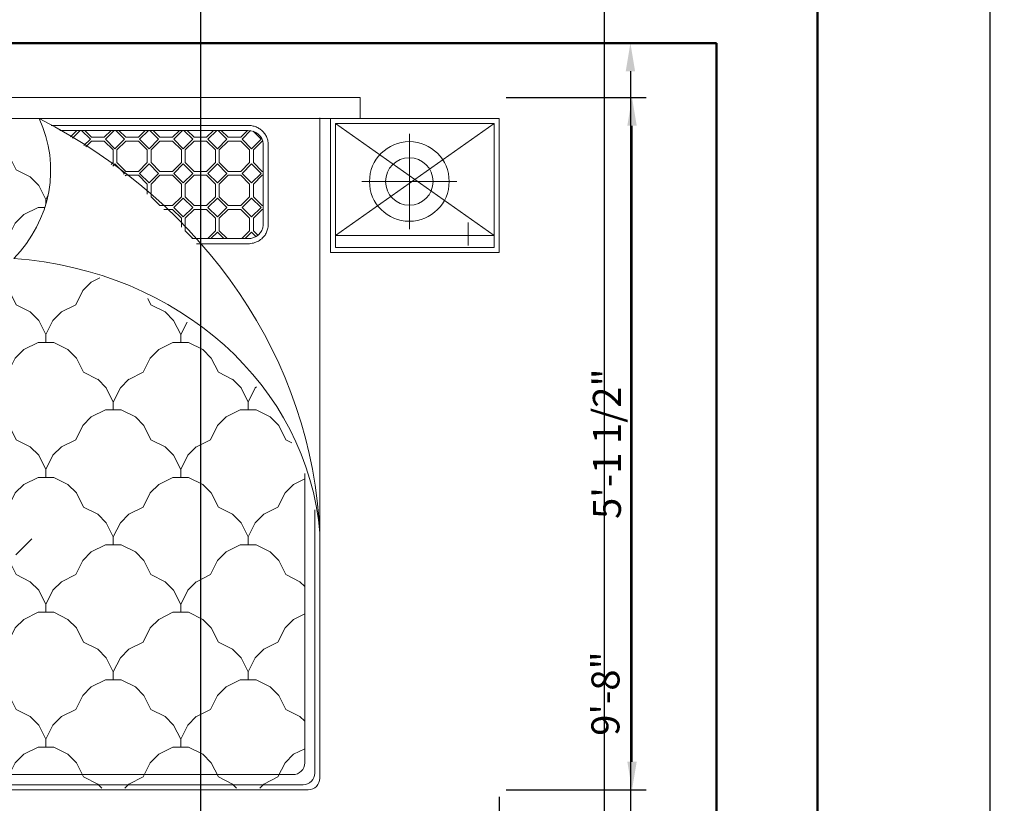
# Model space of a CAD drawing. Units: inches. Extents: x 2385 to 2740, y 1752 to 2305.
# Tile 6 of 15: x 2641 to 2729, y 1911 to 1981. Entities that reach past the tile are written whole.
import ezdxf

# ---------------------------------------------------------------- set-up
doc = ezdxf.new("R2010")
doc.units = ezdxf.units.IN
for name, color, linetype, lineweight in [('A-ANNO-DIMS', 2, 'Continuous', 18), ('A-FURN', 9, 'Continuous', 18), ('A-WALL', 7, 'Continuous', 50)]:
    doc.layers.add(name, color=color, linetype=linetype, lineweight=lineweight)
doc.styles.get("Standard").update_dxf_attribs({"font": 'arial.ttf'})
doc.dimstyles.new('Copy of ISO-25', dxfattribs={"dimtxt": 2.5, "dimasz": 2.5, "dimexe": 1.25, "dimexo": 0.625, "dimtad": 1, "dimdec": 1, "dimlunit": 4, "dimtxsty": 'Standard', "dimcen": 2.5, "dimadec": 0, "dimazin": 0, "dimtfac": 1, "dimtdec": 1, "dimtmove": 0, "dimatfit": 3, "dimfxl": 1, "dimarcsym": 0})

# ---------------------------------------------------------------- blocks, each defined once
blk = doc.blocks.new('A$C029D5C69')
for p, q in [((0.4164, 2.0693), (0.4164, 2.0066)), ((2.2315, 2.0693), (0.4164, 2.0693)), ((2.2315, 2.0066), (2.2315, 2.0693)), ((0, 1.606), (0, 2.0066)), ((0, 2.0066), (0.505, 2.0066)), ((0.4164, 2.0066), (2.2315, 2.0066)), ((0.505, 2.0066), (0.505, 1.606)), ((0.5252, 0.0351), (0.5252, 2.0066)), ((0.5403, 0.0502), (0.5403, 2.0066)), ((0.5706, 0.0805), (0.5706, 2.0066)), ((0.6869, 1.966), (0.6666, 2.0066)), ((0.7072, 2.0066), (0.6869, 1.966)), ((1.0902, 1.966), (1.0699, 2.0066)), ((1.1106, 2.0066), (1.0902, 1.966)), ((2.1114, 2.0087), (2.1114, 0.0351)), ((2.6479, 2.0066), (2.1429, 2.0066)), ((2.1429, 2.0066), (2.1429, 1.606)), ((2.6479, 1.606), (2.6479, 2.0066)), ((0.0151, 1.6211), (0.0151, 1.9915)), ((0.0151, 1.9915), (0.4899, 1.9915)), ((0.4899, 1.9915), (0.4899, 1.6211)), ((1.8954, 1.9865), (1.3081, 1.9865)), ((2.6328, 1.9915), (2.158, 1.9915)), ((2.158, 1.9915), (2.158, 1.6211)), ((2.6328, 1.6211), (2.6328, 1.9915)), ((0.2689, 1.9609), (0.2689, 1.6764)), ((0.6869, 1.9425), (0.6869, 1.966)), ((0.6869, 1.9425), (0.6869, 1.966)), ((1.0902, 1.9425), (1.0902, 1.966)), ((1.0902, 1.9425), (1.0902, 1.966)), ((1.8954, 1.9713), (1.3339, 1.9713)), ((1.3849, 1.9713), (1.3656, 1.952)), ((1.3945, 1.9713), (1.3714, 1.9483)), ((1.4249, 1.945), (1.3986, 1.9713)), ((1.4249, 1.945), (1.4059, 1.926)), ((1.4288, 1.9507), (1.4081, 1.9713)), ((1.4476, 1.9507), (1.4288, 1.9507)), ((1.4476, 1.9507), (1.4664, 1.9507)), ((1.487, 1.9713), (1.4664, 1.9507)), ((1.4966, 1.9713), (1.4703, 1.945)), ((1.4986, 1.9167), (1.4703, 1.945)), ((1.527, 1.945), (1.4986, 1.9167)), ((1.527, 1.945), (1.5007, 1.9713)), ((1.5309, 1.9507), (1.5102, 1.9713)), ((1.5497, 1.9507), (1.5309, 1.9507)), ((1.5497, 1.9507), (1.5685, 1.9507)), ((1.5891, 1.9713), (1.5685, 1.9507)), ((1.5987, 1.9713), (1.5724, 1.945)), ((1.6007, 1.9167), (1.5724, 1.945)), ((1.6291, 1.945), (1.6007, 1.9167)), ((1.6291, 1.945), (1.6028, 1.9713)), ((1.633, 1.9507), (1.6123, 1.9713)), ((1.6518, 1.9507), (1.633, 1.9507)), ((1.6518, 1.9507), (1.6706, 1.9507)), ((1.6912, 1.9713), (1.6706, 1.9507)), ((1.7008, 1.9713), (1.6745, 1.945)), ((1.7028, 1.9167), (1.6745, 1.945)), ((1.7312, 1.945), (1.7028, 1.9167)), ((1.7312, 1.945), (1.7049, 1.9713)), ((1.7351, 1.9507), (1.7144, 1.9713)), ((1.7539, 1.9507), (1.7351, 1.9507)), ((1.7539, 1.9507), (1.7727, 1.9507)), ((1.7933, 1.9713), (1.7727, 1.9507)), ((1.8029, 1.9713), (1.7766, 1.945)), ((1.8049, 1.9167), (1.7766, 1.945)), ((1.8333, 1.945), (1.8049, 1.9167)), ((1.8333, 1.945), (1.807, 1.9713)), ((1.8372, 1.9507), (1.8165, 1.9713)), ((1.856, 1.9507), (1.8372, 1.9507)), ((1.856, 1.9507), (1.8748, 1.9507)), ((1.8954, 1.9713), (1.8748, 1.9507)), ((1.9043, 1.9707), (1.8787, 1.945)), ((1.907, 1.9167), (1.8787, 1.945)), ((1.9354, 1.945), (1.907, 1.9167)), ((1.9354, 1.945), (1.9114, 1.969)), ((2.379, 1.9609), (2.379, 1.6764)), ((0.621, 1.9213), (0.5955, 1.8958)), ((0.6634, 1.9425), (0.621, 1.9213)), ((0.6634, 1.9425), (0.621, 1.9213)), ((0.6869, 1.9425), (0.6634, 1.9425)), ((0.6869, 1.9425), (0.7104, 1.9425)), ((0.7528, 1.9213), (0.7104, 1.9425)), ((0.7528, 1.9213), (0.7104, 1.9425)), ((0.7783, 1.8958), (0.7528, 1.9213)), ((1.0243, 1.9213), (0.9988, 1.8958)), ((1.0668, 1.9425), (1.0244, 1.9213)), ((1.0668, 1.9425), (1.0244, 1.9213)), ((1.0902, 1.9425), (1.0668, 1.9425)), ((1.0902, 1.9425), (1.1137, 1.9425)), ((1.1561, 1.9213), (1.1137, 1.9425)), ((1.1561, 1.9213), (1.1137, 1.9425)), ((1.1816, 1.8958), (1.1561, 1.9213)), ((1.4288, 1.9394), (1.4116, 1.9222)), ((1.4288, 1.9393), (1.4476, 1.9393)), ((1.4664, 1.9393), (1.4476, 1.9393)), ((1.493, 1.9128), (1.4664, 1.9394)), ((1.5309, 1.9394), (1.5043, 1.9128)), ((1.5309, 1.9393), (1.5497, 1.9393)), ((1.5685, 1.9393), (1.5497, 1.9393)), ((1.595, 1.9128), (1.5685, 1.9394)), ((1.633, 1.9394), (1.6064, 1.9128)), ((1.633, 1.9393), (1.6518, 1.9393)), ((1.6706, 1.9393), (1.6518, 1.9393)), ((1.6971, 1.9128), (1.6706, 1.9394)), ((1.7351, 1.9394), (1.7085, 1.9128)), ((1.7351, 1.9393), (1.7539, 1.9393)), ((1.7727, 1.9393), (1.7539, 1.9393)), ((1.7992, 1.9128), (1.7727, 1.9394)), ((1.8372, 1.9394), (1.8106, 1.9128)), ((1.8372, 1.9393), (1.856, 1.9393)), ((1.8748, 1.9393), (1.856, 1.9393)), ((1.9013, 1.9128), (1.8748, 1.9394)), ((1.9393, 1.9394), (1.9127, 1.9128)), ((1.9393, 1.9393), (1.9404, 1.9393)), ((1.9414, 1.688), (1.9414, 1.931)), ((1.9565, 1.688), (1.9565, 1.931)), ((0.5955, 1.8958), (0.5743, 1.8534)), ((0.7995, 1.8534), (0.7783, 1.8958)), ((0.9989, 1.8958), (0.9777, 1.8534)), ((1.2028, 1.8534), (1.1816, 1.8958)), ((1.493, 1.8752), (1.493, 1.9128)), ((1.5043, 1.8752), (1.5043, 1.9128)), ((1.595, 1.8752), (1.595, 1.9128)), ((1.6064, 1.8752), (1.6064, 1.9128)), ((1.6971, 1.8752), (1.6971, 1.9128)), ((1.7085, 1.8752), (1.7085, 1.9128)), ((1.7992, 1.8752), (1.7992, 1.9128)), ((1.8106, 1.8752), (1.8106, 1.9128)), ((1.9013, 1.8752), (1.9013, 1.9128)), ((1.9127, 1.8752), (1.9127, 1.9128)), ((1.493, 1.8752), (1.4867, 1.869)), ((1.4986, 1.8713), (1.4922, 1.8648)), ((1.527, 1.8429), (1.4986, 1.8713)), ((1.5309, 1.8486), (1.5043, 1.8752)), ((1.595, 1.8752), (1.5685, 1.8486)), ((1.6007, 1.8713), (1.5724, 1.8429)), ((1.6291, 1.8429), (1.6007, 1.8713)), ((1.633, 1.8486), (1.6064, 1.8752)), ((1.6971, 1.8752), (1.6706, 1.8486)), ((1.7028, 1.8713), (1.6745, 1.8429)), ((1.7312, 1.8429), (1.7028, 1.8713)), ((1.7351, 1.8486), (1.7085, 1.8752)), ((1.7992, 1.8752), (1.7727, 1.8486)), ((1.8049, 1.8713), (1.7766, 1.8429)), ((1.8333, 1.8429), (1.8049, 1.8713)), ((1.8372, 1.8486), (1.8106, 1.8752)), ((1.9013, 1.8752), (1.8748, 1.8486)), ((1.907, 1.8713), (1.8787, 1.8429)), ((1.9354, 1.8429), (1.907, 1.8713)), ((1.9393, 1.8486), (1.9127, 1.8752)), ((0.5743, 1.8534), (0.5706, 1.8515)), ((0.5743, 1.8534), (0.5706, 1.8515)), ((0.8419, 1.8322), (0.7995, 1.8534)), ((0.8419, 1.8322), (0.7995, 1.8534)), ((0.8674, 1.8067), (0.8419, 1.8322)), ((0.9352, 1.8322), (0.9097, 1.8067)), ((0.9777, 1.8534), (0.9353, 1.8322)), ((0.9777, 1.8534), (0.9353, 1.8322)), ((1.2452, 1.8322), (1.2028, 1.8534)), ((1.2452, 1.8322), (1.2028, 1.8534)), ((1.2707, 1.8067), (1.2452, 1.8322)), ((1.527, 1.8429), (1.5242, 1.8401)), ((1.5309, 1.8373), (1.5295, 1.8359)), ((1.5497, 1.8486), (1.5309, 1.8486)), ((1.5309, 1.8373), (1.5497, 1.8373)), ((1.5497, 1.8486), (1.5685, 1.8486)), ((1.5685, 1.8373), (1.5497, 1.8373)), ((1.595, 1.8107), (1.5685, 1.8373)), ((1.6007, 1.8146), (1.5724, 1.8429)), ((1.6291, 1.8429), (1.6007, 1.8146)), ((1.633, 1.8373), (1.6064, 1.8107)), ((1.6518, 1.8486), (1.633, 1.8486)), ((1.633, 1.8373), (1.6518, 1.8373)), ((1.6518, 1.8486), (1.6706, 1.8486)), ((1.6706, 1.8373), (1.6518, 1.8373)), ((1.6971, 1.8107), (1.6706, 1.8373)), ((1.7028, 1.8146), (1.6745, 1.8429)), ((1.7312, 1.8429), (1.7028, 1.8146)), ((1.7351, 1.8373), (1.7085, 1.8107)), ((1.7539, 1.8486), (1.7351, 1.8486)), ((1.7351, 1.8373), (1.7539, 1.8373)), ((1.7539, 1.8486), (1.7727, 1.8486)), ((1.7727, 1.8373), (1.7539, 1.8373)), ((1.7992, 1.8107), (1.7727, 1.8373)), ((1.8049, 1.8146), (1.7766, 1.8429)), ((1.8333, 1.8429), (1.8049, 1.8146)), ((1.8372, 1.8373), (1.8106, 1.8107)), ((1.856, 1.8486), (1.8372, 1.8486)), ((1.8372, 1.8373), (1.856, 1.8373)), ((1.856, 1.8486), (1.8748, 1.8486)), ((1.8748, 1.8373), (1.856, 1.8373)), ((1.9013, 1.8107), (1.8748, 1.8373)), ((1.907, 1.8146), (1.8787, 1.8429)), ((1.9354, 1.8429), (1.907, 1.8146)), ((1.9393, 1.8373), (1.9127, 1.8107)), ((1.9414, 1.8486), (1.9393, 1.8486)), ((1.9393, 1.8373), (1.9414, 1.8373)), ((0.1267, 1.8186), (0.4111, 1.8186)), ((0.8886, 1.7643), (0.8674, 1.8067)), ((0.9098, 1.8067), (0.8886, 1.7643)), ((1.2919, 1.7643), (1.2707, 1.8067)), ((1.595, 1.7806), (1.595, 1.8107)), ((1.6064, 1.7731), (1.6064, 1.8107)), ((1.6971, 1.7731), (1.6971, 1.8107)), ((1.7085, 1.7731), (1.7085, 1.8107)), ((1.7992, 1.7731), (1.7992, 1.8107)), ((1.8106, 1.7731), (1.8106, 1.8107)), ((1.9013, 1.7731), (1.9013, 1.8107)), ((1.9127, 1.7731), (1.9127, 1.8107)), ((2.2367, 1.8186), (2.5212, 1.8186)), ((1.2981, 1.7768), (1.2919, 1.7643)), ((1.633, 1.7465), (1.6064, 1.7731)), ((1.6971, 1.7731), (1.6706, 1.7465)), ((1.7028, 1.7692), (1.6745, 1.7408)), ((1.7312, 1.7408), (1.7028, 1.7692)), ((1.7351, 1.7465), (1.7085, 1.7731)), ((1.7992, 1.7731), (1.7727, 1.7465)), ((1.8049, 1.7692), (1.7766, 1.7408)), ((1.8333, 1.7408), (1.8049, 1.7692)), ((1.8372, 1.7465), (1.8106, 1.7731)), ((1.9013, 1.7731), (1.8748, 1.7465)), ((1.907, 1.7692), (1.8787, 1.7408)), ((1.9354, 1.7408), (1.907, 1.7692)), ((1.9393, 1.7465), (1.9127, 1.7731)), ((0.8651, 1.7408), (0.8227, 1.7196)), ((0.8651, 1.7408), (0.8227, 1.7196)), ((0.912, 1.7408), (0.8651, 1.7408)), ((0.8886, 1.7408), (0.8886, 1.7643)), ((0.9544, 1.7196), (0.912, 1.7408)), ((0.9544, 1.7196), (0.912, 1.7408)), ((1.2684, 1.7408), (1.226, 1.7196)), ((1.2684, 1.7408), (1.226, 1.7196)), ((1.2885, 1.7408), (1.2684, 1.7408)), ((1.2919, 1.7519), (1.2919, 1.7643)), ((1.6518, 1.7465), (1.633, 1.7465)), ((1.6518, 1.7465), (1.6706, 1.7465)), ((1.7028, 1.7125), (1.6745, 1.7408)), ((1.7312, 1.7408), (1.7028, 1.7125)), ((1.7539, 1.7465), (1.7351, 1.7465)), ((1.7539, 1.7465), (1.7727, 1.7465)), ((1.8049, 1.7125), (1.7766, 1.7408)), ((1.8333, 1.7408), (1.8049, 1.7125)), ((1.856, 1.7465), (1.8372, 1.7465)), ((1.856, 1.7465), (1.8748, 1.7465)), ((1.907, 1.7125), (1.8787, 1.7408)), ((1.9354, 1.7408), (1.907, 1.7125)), ((1.9414, 1.7465), (1.9393, 1.7465)), ((0.8227, 1.7196), (0.7972, 1.6941)), ((0.98, 1.6941), (0.9545, 1.7196)), ((1.226, 1.7196), (1.2005, 1.6941)), ((1.6443, 1.7352), (1.6518, 1.7352)), ((1.6706, 1.7352), (1.6518, 1.7352)), ((1.6971, 1.7086), (1.6706, 1.7352)), ((1.6971, 1.682), (1.6971, 1.7086)), ((1.7351, 1.7352), (1.7085, 1.7086)), ((1.7085, 1.671), (1.7085, 1.7086)), ((1.7351, 1.7352), (1.7539, 1.7352)), ((1.7727, 1.7352), (1.7539, 1.7352)), ((1.7992, 1.7086), (1.7727, 1.7352)), ((1.7992, 1.671), (1.7992, 1.7086)), ((1.8372, 1.7352), (1.8106, 1.7086)), ((1.8106, 1.671), (1.8106, 1.7086)), ((1.8372, 1.7352), (1.856, 1.7352)), ((1.8748, 1.7352), (1.856, 1.7352)), ((1.9013, 1.7086), (1.8748, 1.7352)), ((1.9013, 1.671), (1.9013, 1.7086)), ((1.9393, 1.7352), (1.9127, 1.7086)), ((1.9127, 1.671), (1.9127, 1.7086)), ((1.9393, 1.7352), (1.9414, 1.7352)), ((0.5766, 1.6941), (0.5706, 1.7002)), ((0.5978, 1.6517), (0.5766, 1.6941)), ((0.7972, 1.6941), (0.776, 1.6517)), ((1.0011, 1.6517), (0.9799, 1.6941)), ((1.2005, 1.6941), (1.1793, 1.6517)), ((2.5551, 1.6275), (2.5551, 1.696)), ((0.6402, 1.6305), (0.5978, 1.6517)), ((0.6402, 1.6305), (0.5978, 1.6517)), ((0.776, 1.6517), (0.7336, 1.6305)), ((0.776, 1.6517), (0.7336, 1.6305)), ((1.0435, 1.6305), (1.0011, 1.6517)), ((1.0435, 1.6305), (1.0011, 1.6517)), ((1.1793, 1.6517), (1.1369, 1.6305)), ((1.1793, 1.6517), (1.1369, 1.6305)), ((1.7318, 1.6477), (1.7085, 1.671)), ((1.7992, 1.671), (1.7759, 1.6477)), ((1.8049, 1.6671), (1.7855, 1.6477)), ((1.8244, 1.6477), (1.8049, 1.6671)), ((1.8339, 1.6477), (1.8106, 1.671)), ((1.9013, 1.671), (1.878, 1.6477)), ((1.907, 1.6671), (1.8876, 1.6477)), ((1.9202, 1.6539), (1.907, 1.6671)), ((1.926, 1.6577), (1.9127, 1.671)), ((0.4899, 1.6211), (0.0151, 1.6211)), ((0.6657, 1.605), (0.6402, 1.6305)), ((0.7336, 1.6305), (0.7081, 1.605)), ((1.0691, 1.605), (1.0436, 1.6305)), ((1.1369, 1.6305), (1.1114, 1.605)), ((1.8961, 1.6477), (1.7289, 1.6477)), ((1.8961, 1.6325), (1.7422, 1.6325)), ((2.158, 1.6211), (2.6328, 1.6211)), ((0.505, 1.606), (0, 1.606)), ((0.6869, 1.5626), (0.6657, 1.605)), ((0.7081, 1.605), (0.6869, 1.5626)), ((1.0902, 1.5626), (1.069, 1.605)), ((1.1114, 1.605), (1.0902, 1.5626)), ((2.1429, 1.606), (2.6479, 1.606)), ((0.6869, 1.5392), (0.6869, 1.5626)), ((0.6869, 1.5392), (0.6869, 1.5626)), ((1.0902, 1.5392), (1.0902, 1.5626)), ((1.0902, 1.5392), (1.0902, 1.5626)), ((0.6634, 1.5391), (0.621, 1.5179)), ((0.6634, 1.5391), (0.621, 1.5179)), ((0.6869, 1.5392), (0.6634, 1.5392)), ((0.6869, 1.5392), (0.7104, 1.5392)), ((0.7528, 1.5179), (0.7104, 1.5391)), ((0.7528, 1.5179), (0.7104, 1.5391)), ((1.0668, 1.5391), (1.0244, 1.5179)), ((1.0668, 1.5391), (1.0244, 1.5179)), ((1.0902, 1.5392), (1.0668, 1.5392)), ((1.0902, 1.5392), (1.1137, 1.5392)), ((1.1561, 1.5179), (1.1137, 1.5391)), ((1.1561, 1.5179), (1.1137, 1.5391)), ((0.621, 1.5179), (0.5955, 1.4924)), ((0.7783, 1.4924), (0.7528, 1.5179)), ((1.0243, 1.5179), (0.9988, 1.4924)), ((1.1816, 1.4924), (1.1561, 1.5179)), ((1.4277, 1.5179), (1.4022, 1.4924)), ((1.4534, 1.5308), (1.4277, 1.5179)), ((1.4534, 1.5308), (1.4277, 1.5179)), ((0.5955, 1.4925), (0.5743, 1.4501)), ((0.7995, 1.4501), (0.7783, 1.4925)), ((0.9989, 1.4925), (0.9777, 1.4501)), ((1.2028, 1.4501), (1.1816, 1.4925)), ((1.4022, 1.4925), (1.381, 1.4501)), ((0.5743, 1.45), (0.5706, 1.4481)), ((0.5743, 1.45), (0.5706, 1.4481)), ((0.8419, 1.4288), (0.7995, 1.45)), ((0.8419, 1.4288), (0.7995, 1.45)), ((0.9777, 1.45), (0.9353, 1.4288)), ((0.9777, 1.45), (0.9353, 1.4288)), ((1.2452, 1.4288), (1.2028, 1.45)), ((1.2452, 1.4288), (1.2028, 1.45)), ((1.381, 1.45), (1.3386, 1.4288)), ((1.381, 1.45), (1.3386, 1.4288)), ((1.6062, 1.4501), (1.5966, 1.4692)), ((1.6486, 1.4288), (1.6062, 1.45)), ((1.6486, 1.4288), (1.6062, 1.45)), ((0.8674, 1.4033), (0.8419, 1.4288)), ((0.9352, 1.4288), (0.9097, 1.4033)), ((1.2707, 1.4033), (1.2452, 1.4288)), ((1.3386, 1.4288), (1.3131, 1.4033)), ((1.6741, 1.4033), (1.6486, 1.4288)), ((0.5403, 1.4117), (0.5706, 1.4117)), ((0.8886, 1.361), (0.8674, 1.4034)), ((0.9098, 1.4034), (0.8886, 1.361)), ((1.2919, 1.361), (1.2707, 1.4034)), ((1.3131, 1.4034), (1.2919, 1.361)), ((1.6953, 1.361), (1.6741, 1.4034)), ((1.714, 1.3984), (1.6953, 1.361)), ((0.8886, 1.3375), (0.8886, 1.3609)), ((1.2919, 1.3375), (1.2919, 1.3609)), ((1.6953, 1.3375), (1.6953, 1.3609)), ((0.8651, 1.3374), (0.8227, 1.3162)), ((0.8651, 1.3374), (0.8227, 1.3162)), ((0.912, 1.3375), (0.8651, 1.3375)), ((0.9544, 1.3162), (0.912, 1.3374)), ((0.9544, 1.3162), (0.912, 1.3374)), ((1.2684, 1.3374), (1.226, 1.3162)), ((1.2684, 1.3374), (1.226, 1.3162)), ((1.3154, 1.3375), (1.2684, 1.3375)), ((1.3578, 1.3162), (1.3154, 1.3374)), ((1.3578, 1.3162), (1.3154, 1.3374)), ((1.6718, 1.3374), (1.6294, 1.3162)), ((1.6718, 1.3374), (1.6294, 1.3162)), ((1.7187, 1.3375), (1.6718, 1.3375)), ((1.7611, 1.3162), (1.7187, 1.3374)), ((1.7611, 1.3162), (1.7187, 1.3374)), ((0.5766, 1.2908), (0.5706, 1.2968)), ((0.8227, 1.3163), (0.7972, 1.2908)), ((0.98, 1.2908), (0.9545, 1.3163)), ((1.226, 1.3163), (1.2005, 1.2908)), ((1.3833, 1.2908), (1.3578, 1.3163)), ((1.6294, 1.3163), (1.6039, 1.2908)), ((1.7867, 1.2908), (1.7611, 1.3163)), ((0.5978, 1.2484), (0.5766, 1.2908)), ((0.7972, 1.2908), (0.776, 1.2484)), ((1.0011, 1.2484), (0.9799, 1.2908)), ((1.2005, 1.2908), (1.1793, 1.2484)), ((1.4045, 1.2484), (1.3833, 1.2908)), ((1.6039, 1.2908), (1.5827, 1.2484)), ((1.8078, 1.2484), (1.7866, 1.2908)), ((0.6402, 1.2271), (0.5978, 1.2483)), ((0.6402, 1.2271), (0.5978, 1.2483)), ((0.776, 1.2483), (0.7336, 1.2271)), ((0.776, 1.2483), (0.7336, 1.2271)), ((1.0435, 1.2271), (1.0011, 1.2483)), ((1.0435, 1.2271), (1.0011, 1.2483)), ((1.1793, 1.2483), (1.1369, 1.2271)), ((1.1793, 1.2483), (1.1369, 1.2271)), ((1.4469, 1.2271), (1.4045, 1.2483)), ((1.4469, 1.2271), (1.4045, 1.2483)), ((1.5827, 1.2483), (1.5403, 1.2271)), ((1.5827, 1.2483), (1.5403, 1.2271)), ((1.8502, 1.2271), (1.8078, 1.2483)), ((1.8502, 1.2271), (1.8078, 1.2483)), ((0.5403, 1.21), (0.5706, 1.21)), ((0.6657, 1.2017), (0.6402, 1.2272)), ((0.7336, 1.2272), (0.7081, 1.2017)), ((1.0691, 1.2017), (1.0436, 1.2272)), ((1.1369, 1.2272), (1.1114, 1.2017)), ((1.4724, 1.2017), (1.4469, 1.2272)), ((1.5403, 1.2272), (1.5148, 1.2017)), ((1.8758, 1.2017), (1.8503, 1.2272)), ((0.6869, 1.1593), (0.6657, 1.2017)), ((0.7081, 1.2017), (0.6869, 1.1593)), ((1.0902, 1.1593), (1.069, 1.2017)), ((1.1114, 1.2017), (1.0902, 1.1593)), ((1.4936, 1.1593), (1.4724, 1.2017)), ((1.5148, 1.2017), (1.4936, 1.1593)), ((1.8969, 1.1593), (1.8757, 1.2017)), ((1.9181, 1.2017), (1.8969, 1.1593)), ((1.9215, 1.2051), (1.9181, 1.2017)), ((0.6869, 1.1358), (0.6869, 1.1593)), ((0.6869, 1.1358), (0.6869, 1.1593)), ((1.0902, 1.1358), (1.0902, 1.1593)), ((1.0902, 1.1358), (1.0902, 1.1593)), ((1.4936, 1.1358), (1.4936, 1.1593)), ((1.4936, 1.1358), (1.4936, 1.1593)), ((1.8969, 1.1358), (1.8969, 1.1593)), ((1.8969, 1.1358), (1.8969, 1.1593)), ((0.6634, 1.1358), (0.621, 1.1146)), ((0.6634, 1.1358), (0.621, 1.1146)), ((0.6869, 1.1358), (0.6634, 1.1358)), ((0.6869, 1.1358), (0.7104, 1.1358)), ((0.7528, 1.1146), (0.7104, 1.1358)), ((0.7528, 1.1146), (0.7104, 1.1358)), ((1.0668, 1.1358), (1.0244, 1.1146)), ((1.0668, 1.1358), (1.0244, 1.1146)), ((1.0902, 1.1358), (1.0668, 1.1358)), ((1.0902, 1.1358), (1.1137, 1.1358)), ((1.1561, 1.1146), (1.1137, 1.1358)), ((1.1561, 1.1146), (1.1137, 1.1358)), ((1.4701, 1.1358), (1.4277, 1.1146)), ((1.4701, 1.1358), (1.4277, 1.1146)), ((1.4936, 1.1358), (1.4701, 1.1358)), ((1.4936, 1.1358), (1.5171, 1.1358)), ((1.5595, 1.1146), (1.5171, 1.1358)), ((1.5595, 1.1146), (1.5171, 1.1358)), ((1.8735, 1.1358), (1.8311, 1.1146)), ((1.8735, 1.1358), (1.8311, 1.1146)), ((1.8969, 1.1358), (1.8735, 1.1358)), ((1.8969, 1.1358), (1.9204, 1.1358)), ((1.9628, 1.1146), (1.9204, 1.1358)), ((1.9628, 1.1146), (1.9204, 1.1358)), ((0.621, 1.1146), (0.5955, 1.0891)), ((0.7783, 1.0891), (0.7528, 1.1146)), ((1.0243, 1.1146), (0.9988, 1.0891)), ((1.1816, 1.0891), (1.1561, 1.1146)), ((1.4277, 1.1146), (1.4022, 1.0891)), ((1.585, 1.0891), (1.5595, 1.1146)), ((1.831, 1.1146), (1.8055, 1.0891)), ((1.9883, 1.0891), (1.9628, 1.1146)), ((0.5955, 1.0891), (0.5743, 1.0467)), ((0.7995, 1.0467), (0.7783, 1.0891)), ((0.9989, 1.0891), (0.9777, 1.0467)), ((1.2028, 1.0467), (1.1816, 1.0891)), ((1.4022, 1.0891), (1.381, 1.0467)), ((1.6062, 1.0467), (1.585, 1.0891)), ((1.8056, 1.0891), (1.7844, 1.0467)), ((2.0095, 1.0467), (1.9883, 1.0891)), ((0.5743, 1.0467), (0.5706, 1.0448)), ((0.5743, 1.0467), (0.5706, 1.0448)), ((0.8419, 1.0255), (0.7995, 1.0467)), ((0.8419, 1.0255), (0.7995, 1.0467)), ((0.9777, 1.0467), (0.9353, 1.0255)), ((0.9777, 1.0467), (0.9353, 1.0255)), ((1.2452, 1.0255), (1.2028, 1.0467)), ((1.2452, 1.0255), (1.2028, 1.0467)), ((1.381, 1.0467), (1.3386, 1.0255)), ((1.381, 1.0467), (1.3386, 1.0255)), ((1.6486, 1.0255), (1.6062, 1.0467)), ((1.6486, 1.0255), (1.6062, 1.0467)), ((1.7844, 1.0467), (1.742, 1.0255)), ((1.7844, 1.0467), (1.742, 1.0255)), ((2.0276, 1.0376), (2.0095, 1.0467)), ((2.0276, 1.0376), (2.0095, 1.0467)), ((0.8674, 1), (0.8419, 1.0255)), ((0.9352, 1.0255), (0.9097, 1)), ((1.2707, 1), (1.2452, 1.0255)), ((1.3386, 1.0255), (1.3131, 1)), ((1.6741, 1), (1.6486, 1.0255)), ((1.7419, 1.0255), (1.7164, 1)), ((0.8886, 0.9576), (0.8674, 1)), ((0.9098, 1), (0.8886, 0.9576)), ((1.2919, 0.9576), (1.2707, 1)), ((1.3131, 1), (1.2919, 0.9576)), ((1.6953, 0.9576), (1.6741, 1)), ((1.7165, 1), (1.6953, 0.9576)), ((0.8886, 0.9341), (0.8886, 0.9576)), ((1.2919, 0.9341), (1.2919, 0.9576)), ((1.6953, 0.9341), (1.6953, 0.9576)), ((2.066, 0.9457), (2.066, 0.0805)), ((0.8651, 0.9341), (0.8227, 0.9129)), ((0.8651, 0.9341), (0.8227, 0.9129)), ((0.912, 0.9341), (0.8651, 0.9341)), ((0.9544, 0.9129), (0.912, 0.9341)), ((0.9544, 0.9129), (0.912, 0.9341)), ((1.2684, 0.9341), (1.226, 0.9129)), ((1.2684, 0.9341), (1.226, 0.9129)), ((1.3154, 0.9341), (1.2684, 0.9341)), ((1.3578, 0.9129), (1.3154, 0.9341)), ((1.3578, 0.9129), (1.3154, 0.9341)), ((1.6718, 0.9341), (1.6294, 0.9129)), ((1.6718, 0.9341), (1.6294, 0.9129)), ((1.7187, 0.9341), (1.6718, 0.9341)), ((1.7611, 0.9129), (1.7187, 0.9341)), ((1.7611, 0.9129), (1.7187, 0.9341)), ((2.066, 0.9295), (2.0327, 0.9129)), ((2.066, 0.9295), (2.0327, 0.9129)), ((0.5766, 0.8874), (0.5706, 0.8935)), ((0.5978, 0.845), (0.5766, 0.8874)), ((0.7972, 0.8874), (0.776, 0.845)), ((0.8227, 0.9129), (0.7972, 0.8874)), ((0.98, 0.8874), (0.9545, 0.9129)), ((1.0011, 0.845), (0.9799, 0.8874)), ((1.2005, 0.8874), (1.1793, 0.845)), ((1.226, 0.9129), (1.2005, 0.8874)), ((1.3833, 0.8874), (1.3578, 0.9129)), ((1.4045, 0.845), (1.3833, 0.8874)), ((1.6039, 0.8874), (1.5827, 0.845)), ((1.6294, 0.9129), (1.6039, 0.8874)), ((1.7867, 0.8874), (1.7611, 0.9129)), ((1.8078, 0.845), (1.7866, 0.8874)), ((2.0072, 0.8874), (1.986, 0.845)), ((2.0327, 0.9129), (2.0072, 0.8874)), ((0.6402, 0.8238), (0.5978, 0.845)), ((0.6402, 0.8238), (0.5978, 0.845)), ((0.776, 0.845), (0.7336, 0.8238)), ((0.776, 0.845), (0.7336, 0.8238)), ((1.0435, 0.8238), (1.0011, 0.845)), ((1.0435, 0.8238), (1.0011, 0.845)), ((1.1793, 0.845), (1.1369, 0.8238)), ((1.1793, 0.845), (1.1369, 0.8238)), ((1.4469, 0.8238), (1.4045, 0.845)), ((1.4469, 0.8238), (1.4045, 0.845)), ((1.5827, 0.845), (1.5403, 0.8238)), ((1.5827, 0.845), (1.5403, 0.8238)), ((1.8502, 0.8238), (1.8078, 0.845)), ((1.8502, 0.8238), (1.8078, 0.845)), ((1.986, 0.845), (1.9436, 0.8238)), ((1.986, 0.845), (1.9436, 0.8238)), ((2.0962, 0.8369), (2.0962, 0.0502)), ((0.6657, 0.7983), (0.6402, 0.8238)), ((0.6869, 0.7559), (0.6657, 0.7983)), ((0.7081, 0.7983), (0.6869, 0.7559)), ((0.7336, 0.8238), (0.7081, 0.7983)), ((1.0691, 0.7983), (1.0436, 0.8238)), ((1.0902, 0.7559), (1.069, 0.7983)), ((1.1114, 0.7983), (1.0902, 0.7559)), ((1.1369, 0.8238), (1.1114, 0.7983)), ((1.4724, 0.7983), (1.4469, 0.8238)), ((1.4936, 0.7559), (1.4724, 0.7983)), ((1.5148, 0.7983), (1.4936, 0.7559)), ((1.5403, 0.8238), (1.5148, 0.7983)), ((1.8758, 0.7983), (1.8503, 0.8238)), ((1.8969, 0.7559), (1.8757, 0.7983)), ((1.9181, 0.7983), (1.8969, 0.7559)), ((1.9436, 0.8238), (1.9181, 0.7983)), ((0.6869, 0.7325), (0.6869, 0.7559)), ((0.6869, 0.7325), (0.6869, 0.7559)), ((1.0902, 0.7325), (1.0902, 0.7559)), ((1.0902, 0.7325), (1.0902, 0.7559)), ((1.2024, 0.7028), (1.2503, 0.7507)), ((1.4936, 0.7325), (1.4936, 0.7559)), ((1.4936, 0.7325), (1.4936, 0.7559)), ((1.8969, 0.7325), (1.8969, 0.7559)), ((1.8969, 0.7325), (1.8969, 0.7559)), ((0.621, 0.7113), (0.5955, 0.6858)), ((0.6634, 0.7324), (0.621, 0.7112)), ((0.6634, 0.7324), (0.621, 0.7112)), ((0.6869, 0.7325), (0.6634, 0.7325)), ((0.6869, 0.7325), (0.7104, 0.7325)), ((0.7528, 0.7112), (0.7104, 0.7324)), ((0.7528, 0.7112), (0.7104, 0.7324)), ((0.7783, 0.6858), (0.7528, 0.7113)), ((1.0243, 0.7113), (0.9988, 0.6858)), ((1.0668, 0.7324), (1.0244, 0.7112)), ((1.0668, 0.7324), (1.0244, 0.7112)), ((1.0902, 0.7325), (1.0668, 0.7325)), ((1.0902, 0.7325), (1.1137, 0.7325)), ((1.1561, 0.7112), (1.1137, 0.7324)), ((1.1561, 0.7112), (1.1137, 0.7324)), ((1.1816, 0.6858), (1.1561, 0.7113)), ((1.4277, 0.7113), (1.4022, 0.6858)), ((1.4701, 0.7324), (1.4277, 0.7112)), ((1.4701, 0.7324), (1.4277, 0.7112)), ((1.4936, 0.7325), (1.4701, 0.7325)), ((1.4936, 0.7325), (1.5171, 0.7325)), ((1.5595, 0.7112), (1.5171, 0.7324)), ((1.5595, 0.7112), (1.5171, 0.7324)), ((1.585, 0.6858), (1.5595, 0.7113)), ((1.831, 0.7113), (1.8055, 0.6858)), ((1.8735, 0.7324), (1.8311, 0.7112)), ((1.8735, 0.7324), (1.8311, 0.7112)), ((1.8969, 0.7325), (1.8735, 0.7325)), ((1.8969, 0.7325), (1.9204, 0.7325)), ((1.9628, 0.7112), (1.9204, 0.7324)), ((1.9628, 0.7112), (1.9204, 0.7324)), ((1.9883, 0.6858), (1.9628, 0.7113)), ((0.5955, 0.6858), (0.5743, 0.6434)), ((0.7995, 0.6434), (0.7783, 0.6858)), ((0.9989, 0.6858), (0.9777, 0.6434)), ((1.2028, 0.6434), (1.1816, 0.6858)), ((1.4022, 0.6858), (1.381, 0.6434)), ((1.6062, 0.6434), (1.585, 0.6858)), ((1.8056, 0.6858), (1.7844, 0.6434)), ((2.0095, 0.6434), (1.9883, 0.6858)), ((0.5743, 0.6433), (0.5706, 0.6414)), ((0.5743, 0.6433), (0.5706, 0.6414)), ((0.8419, 0.6221), (0.7995, 0.6433)), ((0.8419, 0.6221), (0.7995, 0.6433)), ((0.8674, 0.5967), (0.8419, 0.6222)), ((0.9352, 0.6222), (0.9097, 0.5967)), ((0.9777, 0.6433), (0.9353, 0.6221)), ((0.9777, 0.6433), (0.9353, 0.6221)), ((1.2452, 0.6221), (1.2028, 0.6433)), ((1.2452, 0.6221), (1.2028, 0.6433)), ((1.2707, 0.5967), (1.2452, 0.6222)), ((1.3386, 0.6222), (1.3131, 0.5967)), ((1.381, 0.6433), (1.3386, 0.6221)), ((1.381, 0.6433), (1.3386, 0.6221)), ((1.6486, 0.6221), (1.6062, 0.6433)), ((1.6486, 0.6221), (1.6062, 0.6433)), ((1.6741, 0.5967), (1.6486, 0.6222)), ((1.7419, 0.6222), (1.7164, 0.5967)), ((1.7844, 0.6433), (1.742, 0.6221)), ((1.7844, 0.6433), (1.742, 0.6221)), ((2.0519, 0.6221), (2.0095, 0.6433)), ((2.0519, 0.6221), (2.0095, 0.6433)), ((2.066, 0.6081), (2.0519, 0.6222)), ((0.8886, 0.5543), (0.8674, 0.5967)), ((0.9098, 0.5967), (0.8886, 0.5543)), ((1.2919, 0.5543), (1.2707, 0.5967)), ((1.3131, 0.5967), (1.2919, 0.5543)), ((1.6953, 0.5543), (1.6741, 0.5967)), ((1.7165, 0.5967), (1.6953, 0.5543)), ((0.8651, 0.5308), (0.8227, 0.5096)), ((0.8651, 0.5308), (0.8227, 0.5096)), ((0.912, 0.5308), (0.8651, 0.5308)), ((0.8886, 0.5308), (0.8886, 0.5543)), ((0.9544, 0.5096), (0.912, 0.5308)), ((0.9544, 0.5096), (0.912, 0.5308)), ((1.2684, 0.5308), (1.226, 0.5096)), ((1.2684, 0.5308), (1.226, 0.5096)), ((1.3154, 0.5308), (1.2684, 0.5308)), ((1.2919, 0.5308), (1.2919, 0.5543)), ((1.3578, 0.5096), (1.3154, 0.5308)), ((1.3578, 0.5096), (1.3154, 0.5308)), ((1.6718, 0.5308), (1.6294, 0.5096)), ((1.6718, 0.5308), (1.6294, 0.5096)), ((1.7187, 0.5308), (1.6718, 0.5308)), ((1.6953, 0.5308), (1.6953, 0.5543)), ((1.7611, 0.5096), (1.7187, 0.5308)), ((1.7611, 0.5096), (1.7187, 0.5308)), ((0.8227, 0.5096), (0.7972, 0.4841)), ((0.98, 0.4841), (0.9545, 0.5096)), ((1.226, 0.5096), (1.2005, 0.4841)), ((1.3833, 0.4841), (1.3578, 0.5096)), ((1.6294, 0.5096), (1.6039, 0.4841)), ((1.7867, 0.4841), (1.7611, 0.5096)), ((2.0327, 0.5096), (2.0072, 0.4841)), ((2.066, 0.5262), (2.0327, 0.5096)), ((2.066, 0.5262), (2.0327, 0.5096)), ((0.5766, 0.4841), (0.5706, 0.4901)), ((0.5978, 0.4417), (0.5766, 0.4841)), ((0.7972, 0.4841), (0.776, 0.4417)), ((1.0011, 0.4417), (0.9799, 0.4841)), ((1.2005, 0.4841), (1.1793, 0.4417)), ((1.4045, 0.4417), (1.3833, 0.4841)), ((1.6039, 0.4841), (1.5827, 0.4417)), ((1.8078, 0.4417), (1.7866, 0.4841)), ((2.0072, 0.4841), (1.986, 0.4417)), ((0.6402, 0.4205), (0.5978, 0.4417)), ((0.6402, 0.4205), (0.5978, 0.4417)), ((0.6657, 0.395), (0.6402, 0.4205)), ((0.7336, 0.4205), (0.7081, 0.395)), ((0.776, 0.4417), (0.7336, 0.4205)), ((0.776, 0.4417), (0.7336, 0.4205)), ((1.0435, 0.4205), (1.0011, 0.4417)), ((1.0435, 0.4205), (1.0011, 0.4417)), ((1.0691, 0.395), (1.0436, 0.4205)), ((1.1369, 0.4205), (1.1114, 0.395)), ((1.1793, 0.4417), (1.1369, 0.4205)), ((1.1793, 0.4417), (1.1369, 0.4205)), ((1.4469, 0.4205), (1.4045, 0.4417)), ((1.4469, 0.4205), (1.4045, 0.4417)), ((1.4724, 0.395), (1.4469, 0.4205)), ((1.5403, 0.4205), (1.5148, 0.395)), ((1.5827, 0.4417), (1.5403, 0.4205)), ((1.5827, 0.4417), (1.5403, 0.4205)), ((1.8502, 0.4205), (1.8078, 0.4417)), ((1.8502, 0.4205), (1.8078, 0.4417)), ((1.8758, 0.395), (1.8503, 0.4205)), ((1.9436, 0.4205), (1.9181, 0.395)), ((1.986, 0.4417), (1.9436, 0.4205)), ((1.986, 0.4417), (1.9436, 0.4205)), ((0.6869, 0.3526), (0.6657, 0.395)), ((0.7081, 0.395), (0.6869, 0.3526)), ((1.0902, 0.3526), (1.069, 0.395)), ((1.1114, 0.395), (1.0902, 0.3526)), ((1.4936, 0.3526), (1.4724, 0.395)), ((1.5148, 0.395), (1.4936, 0.3526)), ((1.8969, 0.3526), (1.8757, 0.395)), ((1.9181, 0.395), (1.8969, 0.3526)), ((0.6634, 0.3291), (0.621, 0.3079)), ((0.6634, 0.3291), (0.621, 0.3079)), ((0.6869, 0.3291), (0.6634, 0.3291)), ((0.6869, 0.3291), (0.6869, 0.3526)), ((0.6869, 0.3291), (0.6869, 0.3526)), ((0.6869, 0.3291), (0.7104, 0.3291)), ((0.7528, 0.3079), (0.7104, 0.3291)), ((0.7528, 0.3079), (0.7104, 0.3291)), ((1.0668, 0.3291), (1.0244, 0.3079)), ((1.0668, 0.3291), (1.0244, 0.3079)), ((1.0902, 0.3291), (1.0668, 0.3291)), ((1.0902, 0.3291), (1.0902, 0.3526)), ((1.0902, 0.3291), (1.0902, 0.3526)), ((1.0902, 0.3291), (1.1137, 0.3291)), ((1.1561, 0.3079), (1.1137, 0.3291)), ((1.1561, 0.3079), (1.1137, 0.3291)), ((1.4701, 0.3291), (1.4277, 0.3079)), ((1.4701, 0.3291), (1.4277, 0.3079)), ((1.4936, 0.3291), (1.4701, 0.3291)), ((1.4936, 0.3291), (1.4936, 0.3526)), ((1.4936, 0.3291), (1.4936, 0.3526)), ((1.4936, 0.3291), (1.5171, 0.3291)), ((1.5595, 0.3079), (1.5171, 0.3291)), ((1.5595, 0.3079), (1.5171, 0.3291)), ((1.8735, 0.3291), (1.8311, 0.3079)), ((1.8735, 0.3291), (1.8311, 0.3079)), ((1.8969, 0.3291), (1.8735, 0.3291)), ((1.8969, 0.3291), (1.8969, 0.3526)), ((1.8969, 0.3291), (1.8969, 0.3526)), ((1.8969, 0.3291), (1.9204, 0.3291)), ((1.9628, 0.3079), (1.9204, 0.3291)), ((1.9628, 0.3079), (1.9204, 0.3291)), ((0.621, 0.3079), (0.5955, 0.2824)), ((0.7783, 0.2824), (0.7528, 0.3079)), ((1.0243, 0.3079), (0.9988, 0.2824)), ((1.1816, 0.2824), (1.1561, 0.3079)), ((1.4277, 0.3079), (1.4022, 0.2824)), ((1.585, 0.2824), (1.5595, 0.3079)), ((1.831, 0.3079), (1.8055, 0.2824)), ((1.9883, 0.2824), (1.9628, 0.3079)), ((0.5955, 0.2824), (0.5743, 0.24)), ((0.7995, 0.24), (0.7783, 0.2824)), ((0.9989, 0.2824), (0.9777, 0.24)), ((1.2028, 0.24), (1.1816, 0.2824)), ((1.4022, 0.2824), (1.381, 0.24)), ((1.6062, 0.24), (1.585, 0.2824)), ((1.8056, 0.2824), (1.7844, 0.24)), ((2.0095, 0.24), (1.9883, 0.2824)), ((0.5743, 0.24), (0.5706, 0.2381)), ((0.5743, 0.24), (0.5706, 0.2381)), ((0.8419, 0.2188), (0.7995, 0.24)), ((0.8419, 0.2188), (0.7995, 0.24)), ((0.9777, 0.24), (0.9353, 0.2188)), ((0.9777, 0.24), (0.9353, 0.2188)), ((1.2452, 0.2188), (1.2028, 0.24)), ((1.2452, 0.2188), (1.2028, 0.24)), ((1.381, 0.24), (1.3386, 0.2188)), ((1.381, 0.24), (1.3386, 0.2188)), ((1.6486, 0.2188), (1.6062, 0.24)), ((1.6486, 0.2188), (1.6062, 0.24)), ((1.7844, 0.24), (1.742, 0.2188)), ((1.7844, 0.24), (1.742, 0.2188)), ((2.0519, 0.2188), (2.0095, 0.24)), ((2.0519, 0.2188), (2.0095, 0.24)), ((0.8674, 0.1933), (0.8419, 0.2188)), ((0.9352, 0.2188), (0.9097, 0.1933)), ((1.2707, 0.1933), (1.2452, 0.2188)), ((1.3386, 0.2188), (1.3131, 0.1933)), ((1.6741, 0.1933), (1.6486, 0.2188)), ((1.7419, 0.2188), (1.7164, 0.1933)), ((2.066, 0.2047), (2.0519, 0.2188)), ((0.8886, 0.1509), (0.8674, 0.1933)), ((0.9098, 0.1933), (0.8886, 0.1509)), ((1.2919, 0.1509), (1.2707, 0.1933)), ((1.3131, 0.1933), (1.2919, 0.1509)), ((1.6953, 0.1509), (1.6741, 0.1933)), ((1.7165, 0.1933), (1.6953, 0.1509)), ((0.8886, 0.1275), (0.8886, 0.1509)), ((1.2919, 0.1275), (1.2919, 0.1509)), ((1.6953, 0.1275), (1.6953, 0.1509)), ((0.8651, 0.1274), (0.8227, 0.1062)), ((0.8651, 0.1274), (0.8227, 0.1062)), ((0.912, 0.1275), (0.8651, 0.1275)), ((0.9544, 0.1062), (0.912, 0.1274)), ((0.9544, 0.1062), (0.912, 0.1274)), ((1.2684, 0.1274), (1.226, 0.1062)), ((1.2684, 0.1274), (1.226, 0.1062)), ((1.3154, 0.1275), (1.2684, 0.1275)), ((1.3578, 0.1062), (1.3154, 0.1274)), ((1.3578, 0.1062), (1.3154, 0.1274)), ((1.6718, 0.1274), (1.6294, 0.1062)), ((1.6718, 0.1274), (1.6294, 0.1062)), ((1.7187, 0.1275), (1.6718, 0.1275)), ((1.7611, 0.1062), (1.7187, 0.1274)), ((1.7611, 0.1062), (1.7187, 0.1274)), ((2.066, 0.1228), (2.0327, 0.1062)), ((2.066, 0.1228), (2.0327, 0.1062)), ((0.8227, 0.1062), (0.7972, 0.0807)), ((0.98, 0.0807), (0.9545, 0.1062)), ((1.226, 0.1062), (1.2005, 0.0807)), ((1.3833, 0.0807), (1.3578, 0.1062)), ((1.6294, 0.1062), (1.6039, 0.0807)), ((1.7867, 0.0807), (1.7611, 0.1062)), ((2.0327, 0.1062), (2.0072, 0.0807)), ((0.5766, 0.0807), (0.5706, 0.0868)), ((0.5978, 0.0384), (0.5766, 0.0808)), ((0.7972, 0.0808), (0.776, 0.0384)), ((1.0011, 0.0384), (0.9799, 0.0808)), ((1.2005, 0.0808), (1.1793, 0.0384)), ((1.4045, 0.0384), (1.3833, 0.0808)), ((1.6039, 0.0808), (1.5827, 0.0384)), ((1.8078, 0.0384), (1.7866, 0.0808)), ((2.0072, 0.0808), (1.986, 0.0384)), ((0.6402, 0.0171), (0.5978, 0.0383)), ((0.6402, 0.0171), (0.5978, 0.0383)), ((2.0309, 0.0454), (0.6056, 0.0454)), ((0.776, 0.0383), (0.7336, 0.0171)), ((0.776, 0.0383), (0.7336, 0.0171)), ((1.0435, 0.0171), (1.0011, 0.0383)), ((1.0435, 0.0171), (1.0011, 0.0383)), ((1.1793, 0.0383), (1.1369, 0.0171)), ((1.1793, 0.0383), (1.1369, 0.0171)), ((1.4469, 0.0171), (1.4045, 0.0383)), ((1.4469, 0.0171), (1.4045, 0.0383)), ((1.5827, 0.0383), (1.5403, 0.0171)), ((1.5827, 0.0383), (1.5403, 0.0171)), ((1.8502, 0.0171), (1.8078, 0.0383)), ((1.8502, 0.0171), (1.8078, 0.0383)), ((1.986, 0.0383), (1.9436, 0.0171)), ((1.986, 0.0383), (1.9436, 0.0171)), ((2.0763, 0), (0.5603, 0)), ((2.0612, 0.0151), (0.5754, 0.0151)), ((0.6523, 0.005), (0.6402, 0.0171)), ((0.7336, 0.0171), (0.7215, 0.005)), ((1.0557, 0.005), (1.0436, 0.0171)), ((1.1369, 0.0171), (1.1248, 0.005)), ((1.459, 0.005), (1.4469, 0.0171)), ((1.5403, 0.0171), (1.5282, 0.005)), ((1.8623, 0.005), (1.8503, 0.0171)), ((1.9436, 0.0171), (1.9315, 0.005))]:
    blk.add_line(p, q)
at = {"ltscale": 0.005}
for p, q in [((0.4899, 1.6568), (0.0151, 1.9915)), ((0.0151, 1.6568), (0.4899, 1.9915)), ((2.6328, 1.6568), (2.158, 1.9915)), ((2.158, 1.6568), (2.6328, 1.9915)), ((0.0151, 1.6568), (0.4899, 1.6568)), ((2.6328, 1.6568), (2.158, 1.6568))]:
    blk.add_line(p, q, dxfattribs=at)
for centre, radius in [((0.2689, 1.8186), 0.1191), ((2.379, 1.8186), 0.1191), ((0.2689, 1.8186), 0.0711), ((2.379, 1.8186), 0.0711)]:
    blk.add_circle(centre, radius)
for centre, radius, start, end in [((0.2843, 0.0157), 0.6251, 10.2961, 13.2684), ((0.6056, 0.0805), 0.0351, 180, 270), ((2.0309, 0.0805), 0.0351, 270, 0), ((0.5603, 0.0351), 0.0351, 180, 270), ((0.5754, 0.0502), 0.0351, 180, 270), ((2.0612, 0.0502), 0.0351, 270, 0), ((2.0763, 0.0351), 0.0351, 270, 0)]:
    blk.add_arc(centre, radius, start, end)
for centre, major_axis, ratio, start_param, end_param in [((0.8506, 1.8527), (-0.4556, 0), 0.89, 2.430919, 3.53111), ((0.3667, 0.6698), (1.7398, 0.1668), 0.88072, -0.045073, 0.941433), ((1.8961, 1.931), (-0.0453, 0), 0.89, 3.141593, 4.712389), ((1.8961, 1.688), (-0.0453, 0), 0.89, 1.570796, 3.141593), ((1.0874, 0.6748), (1.021, 0.1213), 0.889348, -0.031673, 1.359628)]:
    blk.add_ellipse(centre, major_axis=major_axis, ratio=ratio, start_param=start_param, end_param=end_param)
for points, knots in [([(1.9565, 1.931), (1.9565, 1.9336), (1.9563, 1.9362), (1.9553, 1.9428), (1.9543, 1.9467), (1.9512, 1.9541), (1.9493, 1.9577), (1.9446, 1.9643), (1.942, 1.9674), (1.936, 1.9729), (1.9327, 1.9753), (1.9257, 1.9795), (1.922, 1.9813), (1.9142, 1.9841), (1.9102, 1.9851), (1.9028, 1.9862), (1.8995, 1.9865), (1.8961, 1.9865)], [3.141593, 3.141593, 3.141593, 3.141593, 3.277614, 3.277614, 3.488082, 3.488082, 3.698551, 3.698551, 3.909019, 3.909019, 4.119488, 4.119488, 4.329956, 4.329956, 4.540424, 4.540424, 4.712389, 4.712389, 4.712389, 4.712389]), ([(1.8961, 1.6325), (1.899, 1.6325), (1.9019, 1.6327), (1.9101, 1.6338), (1.9153, 1.6352), (1.9253, 1.6392), (1.93, 1.6418), (1.9385, 1.6481), (1.9423, 1.6519), (1.9481, 1.6594), (1.9503, 1.663), (1.9537, 1.6707), (1.955, 1.6747), (1.9563, 1.6818), (1.9565, 1.6849), (1.9565, 1.688)], [1.570796, 1.570796, 1.570796, 1.570796, 1.718836, 1.718836, 1.993452, 1.993452, 2.268068, 2.268068, 2.542684, 2.542684, 2.761386, 2.761386, 2.980087, 2.980087, 3.141593, 3.141593, 3.141593, 3.141593])]:
    blk.add_open_spline(points, degree=3, knots=knots)
blk = doc.blocks.new('*D17')
at = {"layer": 'A-ANNO-DIMS', "color": 0, "lineweight": -2, "transparency": 16777216}
for p, q in [((2702.623, 1978.97), (2694.318, 1978.97)), ((2695.568, 1976.47), (2695.568, 1865.47)), ((2702.623, 1862.97), (2694.318, 1862.97))]:
    blk.add_line(p, q, dxfattribs=at)
at = {"layer": 'A-ANNO-DIMS', "color": 0, "transparency": 16777216}
for points in [[(2695.152, 1976.47), (2695.985, 1976.47), (2695.568, 1978.97)], [(2695.152, 1865.47), (2695.985, 1865.47), (2695.568, 1862.97)]]:
    blk.add_solid(points, dxfattribs=at)
at = {"layer": 'Defpoints', "color": 0, "transparency": 16777216}
for p in [(2703.248, 1978.97), (2695.568, 1862.97), (2703.248, 1862.97)]:
    blk.add_point(p, dxfattribs=at)
at = {"layer": 'A-ANNO-DIMS', "color": 0, "transparency": 16777216, "insert": (2693.667, 1920.97), "char_height": 2.5, "attachment_point": 5, "rotation": 90}
blk.add_mtext('9\'-8"', dxfattribs=at)
blk = doc.blocks.new('*D25')
at = {"layer": 'A-ANNO-DIMS', "color": 0, "lineweight": -2, "transparency": 16777216}
for p, q in [((2712.873, 2275.97), (2728.926, 2275.97)), ((2727.676, 1781.47), (2727.676, 2273.47)), ((2712.873, 1778.97), (2728.926, 1778.97))]:
    blk.add_line(p, q, dxfattribs=at)
at = {"layer": 'A-ANNO-DIMS', "color": 0, "transparency": 16777216}
for points in [[(2727.259, 2273.47), (2728.092, 2273.47), (2727.676, 2275.97)], [(2727.259, 1781.47), (2728.092, 1781.47), (2727.676, 1778.97)]]:
    blk.add_solid(points, dxfattribs=at)
at = {"layer": 'Defpoints', "color": 0, "transparency": 16777216}
for p in [(2712.248, 2275.97), (2727.676, 2275.97), (2712.248, 1778.97)]:
    blk.add_point(p, dxfattribs=at)
at = {"layer": 'A-ANNO-DIMS', "color": 0, "transparency": 16777216, "insert": (2725.774, 2027.47), "char_height": 2.5, "attachment_point": 5, "rotation": 90}
blk.add_mtext('41\'-5"', dxfattribs=at)
blk = doc.blocks.new('*D28')
at = {"layer": 'A-ANNO-DIMS', "color": 0, "lineweight": -2, "transparency": 16777216}
for p, q in [((2604.89, 1911.766), (2604.89, 1899.294)), ((2683.867, 1911.766), (2683.867, 1899.294)), ((2607.39, 1900.544), (2681.367, 1900.544))]:
    blk.add_line(p, q, dxfattribs=at)
at = {"layer": 'A-ANNO-DIMS', "color": 0, "transparency": 16777216}
for points in [[(2607.39, 1900.961), (2607.39, 1900.127), (2604.89, 1900.544)], [(2681.367, 1900.961), (2681.367, 1900.127), (2683.867, 1900.544)]]:
    blk.add_solid(points, dxfattribs=at)
at = {"layer": 'Defpoints', "color": 0, "transparency": 16777216}
for p in [(2604.89, 1912.391), (2683.867, 1912.391), (2683.867, 1900.544)]:
    blk.add_point(p, dxfattribs=at)
at = {"layer": 'A-ANNO-DIMS', "color": 0, "transparency": 16777216, "insert": (2644.378, 1902.445), "char_height": 2.5, "attachment_point": 5}
blk.add_mtext('BED 6\'-7"', dxfattribs=at)
blk = doc.blocks.new('*D29')
at = {"layer": 'A-ANNO-DIMS', "color": 0, "lineweight": -2, "transparency": 16777216}
for p, q in [((2684.492, 1974.11), (2696.964, 1974.11)), ((2695.714, 1914.891), (2695.714, 1971.61)), ((2684.492, 1912.391), (2696.964, 1912.391))]:
    blk.add_line(p, q, dxfattribs=at)
at = {"layer": 'A-ANNO-DIMS', "color": 0, "transparency": 16777216}
for points in [[(2695.297, 1971.61), (2696.131, 1971.61), (2695.714, 1974.11)], [(2695.297, 1914.891), (2696.131, 1914.891), (2695.714, 1912.391)]]:
    blk.add_solid(points, dxfattribs=at)
at = {"layer": 'Defpoints', "color": 0, "transparency": 16777216}
for p in [(2683.867, 1974.11), (2695.714, 1974.11), (2683.867, 1912.391)]:
    blk.add_point(p, dxfattribs=at)
at = {"layer": 'A-ANNO-DIMS', "color": 0, "transparency": 16777216, "insert": (2693.796, 1943.25), "char_height": 2.5, "attachment_point": 5, "rotation": 90}
blk.add_mtext('5\'-1 1/2"', dxfattribs=at)
blk = doc.blocks.new('*D43')
at = {"layer": 'A-ANNO-DIMS', "color": 0, "lineweight": -2, "transparency": 16777216}
for p, q in [((2657.248, 1863.595), (2657.248, 2302.837)), ((2693.248, 1863.595), (2693.248, 2302.837)), ((2659.748, 2301.587), (2690.748, 2301.587))]:
    blk.add_line(p, q, dxfattribs=at)
at = {"layer": 'A-ANNO-DIMS', "color": 0, "transparency": 16777216}
for points in [[(2659.748, 2302.004), (2659.748, 2301.171), (2657.248, 2301.587)], [(2690.748, 2302.004), (2690.748, 2301.171), (2693.248, 2301.587)]]:
    blk.add_solid(points, dxfattribs=at)
at = {"layer": 'Defpoints', "color": 0, "transparency": 16777216}
for p in [(2693.248, 2301.587), (2657.248, 1862.97), (2693.248, 1862.97)]:
    blk.add_point(p, dxfattribs=at)
at = {"layer": 'A-ANNO-DIMS', "color": 0, "transparency": 16777216, "insert": (2675.248, 2303.49), "char_height": 2.5, "attachment_point": 5}
blk.add_mtext('3\'-0"', dxfattribs=at)

msp = doc.modelspace()

# ---------------------------------------------------------------- linework, layer by layer
at = {"layer": 'A-WALL'}
for p, q in [((2712.248, 2275.97), (2712.248, 1778.97)), ((2712.248, 1984.97), (2712.248, 1978.97)), ((2559.248, 1978.97), (2703.248, 1978.97)), ((2703.248, 1978.97), (2703.248, 1862.97)), ((2703.248, 1978.97), (2703.248, 1862.97)), ((2712.248, 1978.97), (2712.248, 1862.97))]:
    msp.add_line(p, q, dxfattribs=at)

# ---------------------------------------------------------------- block references
at = {"layer": 'A-FURN', "xscale": 29.82667023927314, "yscale": 29.82667023927314, "zscale": 29.82667023927314}
msp.add_blockref('A$C029D5C69', (2604.89, 1912.391), dxfattribs=at)

# ---------------------------------------------------------------- dimensions: what is measured, and where the dimension line sits
at = {"layer": 'A-ANNO-DIMS'}
dim = msp.add_linear_dim(base=(2693.248, 2301.587), p1=(2657.248, 1862.97), p2=(2693.248, 1862.97), dimstyle='Copy of ISO-25', override={"dimdec": 1, "dimlfac": 1, "dimrnd": 0, "dimzin": 1, "dimdsep": 46, "dimlunit": 4, "dimfrac": 2}, dxfattribs=at)
dim.commit()
dim.dimension.update_dxf_attribs({"geometry": '*D43', "text_midpoint": (2675.248, 2303.49)})
for base, p1, p2, override, picture, middle in [((2727.676, 2275.97), (2712.248, 1778.97), (2712.248, 2275.97), {"dimclrd": 0, "dimclre": 0, "dimclrt": 0}, '*D25', (2725.774, 2027.47)), ((2695.568, 1862.97), (2703.248, 1978.97), (2703.248, 1862.97), {"dimclrd": 0, "dimclre": 0, "dimclrt": 0}, '*D17', (2693.667, 1920.97)), ((2695.714, 1974.11), (2683.867, 1912.391), (2683.867, 1974.11), {"dimdec": 1, "dimlfac": 1, "dimrnd": 0, "dimzin": 1, "dimdsep": 46, "dimlunit": 4, "dimfrac": 2}, '*D29', (2693.796, 1943.25))]:
    dim = msp.add_linear_dim(base=base, p1=p1, p2=p2, angle=90, dimstyle='Copy of ISO-25', override=override, dxfattribs=at)
    dim.commit()
    dim.dimension.update_dxf_attribs({"geometry": picture, "text_midpoint": middle})
dim = msp.add_linear_dim(base=(2683.867, 1900.544), p1=(2604.89, 1912.391), p2=(2683.867, 1912.391), text='BED <>', dimstyle='Copy of ISO-25', override={"dimdec": 1, "dimlfac": 1, "dimrnd": 0, "dimzin": 1, "dimdsep": 46, "dimlunit": 4, "dimfrac": 2}, dxfattribs=at)
dim.commit()
dim.dimension.update_dxf_attribs({"geometry": '*D28', "text_midpoint": (2644.378, 1902.445)})

doc.saveas('drawing.dxf')
